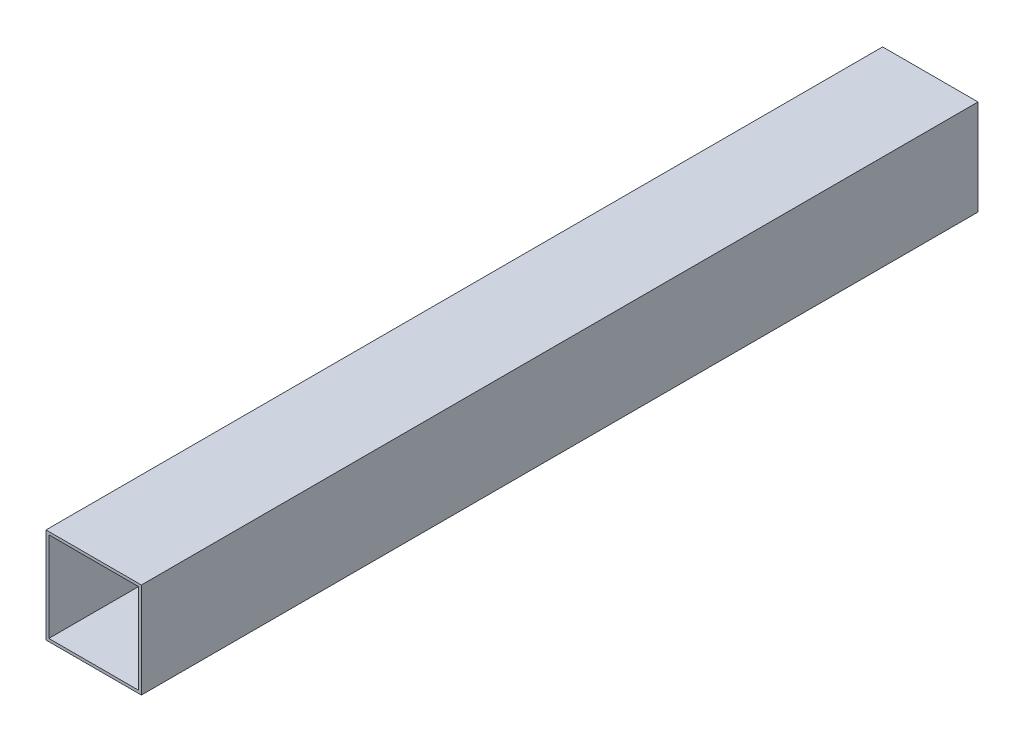
from build123d import *

# Parameters (mm, degrees)
TUBE_PROFILE_8X8_SQUARE_W           = 215.9
TUBE_PROFILE_8X8_SQUARE_H           = 215.9
TUBE_PROFILE_8X8_SQUARE_W_2         = 203.2
TUBE_PROFILE_8X8_SQUARE_H_2         = 203.2
SQUARE_TUBE_8_5X8_5X0_25_WALL_DEPTH = 1893.8875


with BuildPart() as part:
    # Tube Profile 8x8 Square → Square Tube 8.5x8.5x0.25 Wall (new body)
    with BuildSketch(Plane.XY):
        Rectangle(TUBE_PROFILE_8X8_SQUARE_W, TUBE_PROFILE_8X8_SQUARE_H)
        Rectangle(TUBE_PROFILE_8X8_SQUARE_W_2, TUBE_PROFILE_8X8_SQUARE_H_2, mode=Mode.SUBTRACT)
    extrude(amount=SQUARE_TUBE_8_5X8_5X0_25_WALL_DEPTH)


solid = part.part
